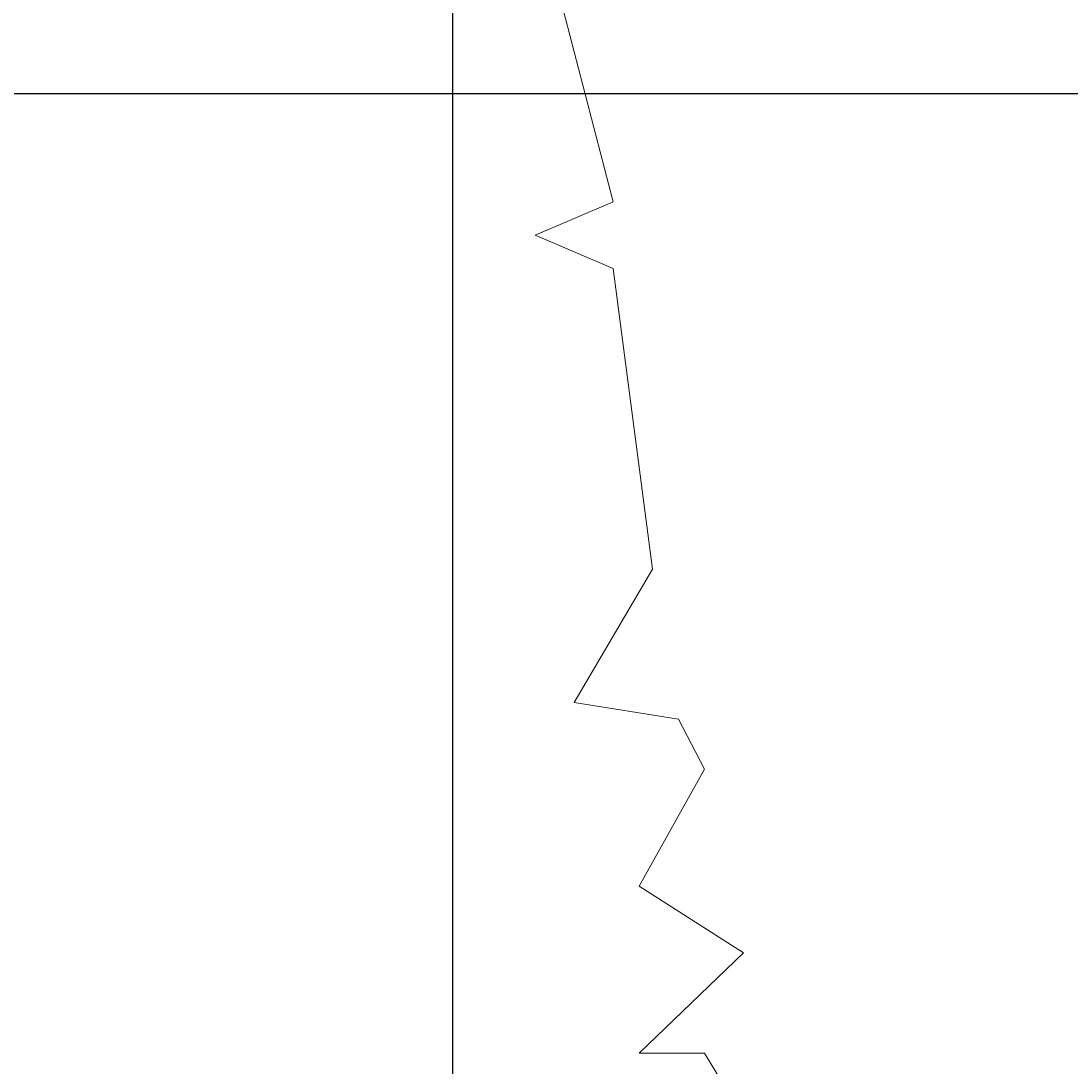
# Model space of a CAD drawing. Units: inches. Extents: x -26 to 776, y -22 to 650.
# Tile 57 of 62: x 506 to 601, y 226 to 321. Entities that reach past the tile are written whole.
import ezdxf

# ---------------------------------------------------------------- set-up
doc = ezdxf.new("R2010")
doc.units = ezdxf.units.IN
doc.header["$MEASUREMENT"] = 0
doc.layers.add('A-ANNO-DIMS', color=2, linetype='Continuous', lineweight=18)
doc.layers.add('L-PLNT-TREE', color=94, linetype='Continuous', lineweight=18)
doc.styles.get("Standard").update_dxf_attribs({"font": 'arial.ttf'})
doc.dimstyles.get("Standard").update_dxf_attribs({"dimtxt": 0.5625, "dimasz": 0.18, "dimexe": 0.18, "dimexo": 0.0625, "dimgap": 0.09, "dimtad": 0, "dimtih": 1, "dimtoh": 1, "dimdec": 4, "dimzin": 0, "dimdsep": 46, "dimlunit": 4, "dimtxsty": 'Standard', "dimcen": 0.09, "dimadec": 0, "dimazin": 0, "dimtfac": 1, "dimtdec": 4, "dimtofl": 0, "dimtmove": 0, "dimatfit": 3, "dimfxl": 1, "dimtolj": 1, "dimtzin": 0, "dimarcsym": 0})

# ---------------------------------------------------------------- blocks, each defined once
blk = doc.blocks.new('Tree - type 2 deciduous elevation')
blk.add_lwpolyline([(34.628, 89.951), (26.576, 103.222), (23.701, 103.222), (28.302, 107.646), (23.701, 110.595), (26.576, 115.756), (25.426, 117.968), (20.825, 118.706), (24.276, 124.604), (22.551, 137.876), (19.1, 139.35), (22.551, 140.825), (19.675, 151.884)])
blk = doc.blocks.new('*D20')
at = {"layer": 'A-ANNO-DIMS', "color": 0, "lineweight": -2, "transparency": 16777216}
for p, q in [((425.806, 455.472), (775.335, 455.472)), ((775.155, 455.292), (775.155, 235.854)), ((775.155, 15.662), (775.155, 235.1)), ((425.806, 15.482), (775.335, 15.482))]:
    blk.add_line(p, q, dxfattribs=at)
at = {"layer": 'A-ANNO-DIMS', "color": 0, "transparency": 16777216}
for points in [[(775.125, 455.292), (775.185, 455.292), (775.155, 455.472)], [(775.125, 15.662), (775.185, 15.662), (775.155, 15.482)]]:
    blk.add_solid(points, dxfattribs=at)
at = {"layer": 'Defpoints', "color": 0, "transparency": 16777216}
for p in [(425.743, 455.472), (775.155, 455.472), (425.743, 15.482)]:
    blk.add_point(p, dxfattribs=at)
at = {"layer": 'A-ANNO-DIMS', "color": 0, "transparency": 16777216, "insert": (775.155, 235.477), "char_height": 0.5625, "attachment_point": 5}
blk.add_mtext('\\A1;440', dxfattribs=at)
blk = doc.blocks.new('*D28')
at = {"layer": 'A-ANNO-DIMS', "color": 0, "lineweight": -2, "transparency": 16777216}
for p, q in [((285.08, 314.119), (775.335, 314.119)), ((775.155, 313.939), (775.155, 243.141)), ((775.155, 171.597), (775.155, 242.396)), ((285.08, 171.417), (775.335, 171.417))]:
    blk.add_line(p, q, dxfattribs=at)
at = {"layer": 'A-ANNO-DIMS', "color": 0, "transparency": 16777216}
for points in [[(775.125, 313.939), (775.185, 313.939), (775.155, 314.119)], [(775.125, 171.597), (775.185, 171.597), (775.155, 171.417)]]:
    blk.add_solid(points, dxfattribs=at)
at = {"layer": 'Defpoints', "color": 0, "transparency": 16777216}
for p in [(285.018, 314.119), (775.155, 314.119), (285.018, 171.417)]:
    blk.add_point(p, dxfattribs=at)
at = {"layer": 'A-ANNO-DIMS', "color": 0, "transparency": 16777216, "insert": (775.155, 242.768), "char_height": 0.5625, "attachment_point": 5}
blk.add_mtext('\\A1;142.7', dxfattribs=at)
blk = doc.blocks.new('*D45')
at = {"layer": 'A-ANNO-DIMS', "color": 0, "lineweight": -2, "transparency": 16777216}
for p, q in [((507.738, 408.639), (775.335, 408.639)), ((775.155, 408.459), (775.155, 212.438)), ((775.155, 15.662), (775.155, 211.683)), ((585.998, 15.482), (775.335, 15.482))]:
    blk.add_line(p, q, dxfattribs=at)
at = {"layer": 'A-ANNO-DIMS', "color": 0, "transparency": 16777216}
for points in [[(775.125, 408.459), (775.185, 408.459), (775.155, 408.639)], [(775.125, 15.662), (775.185, 15.662), (775.155, 15.482)]]:
    blk.add_solid(points, dxfattribs=at)
at = {"layer": 'Defpoints', "color": 0, "transparency": 16777216}
for p in [(507.676, 408.639), (775.155, 408.639), (585.935, 15.482)]:
    blk.add_point(p, dxfattribs=at)
at = {"layer": 'A-ANNO-DIMS', "color": 0, "transparency": 16777216, "insert": (775.155, 212.061), "char_height": 0.5625, "attachment_point": 5}
blk.add_mtext('\\A1;393.16', dxfattribs=at)
blk = doc.blocks.new('*D48')
at = {"layer": 'A-ANNO-DIMS', "color": 0, "lineweight": -2, "transparency": 16777216}
for p, q in [((545.033, 67.415), (545.033, 649.856)), ((545.213, 649.676), (640.879, 649.676)), ((738.57, 649.676), (642.904, 649.676)), ((738.75, 50.911), (738.75, 649.856))]:
    blk.add_line(p, q, dxfattribs=at)
at = {"layer": 'A-ANNO-DIMS', "color": 0, "transparency": 16777216}
for points in [[(545.213, 649.706), (545.213, 649.646), (545.033, 649.676)], [(738.57, 649.706), (738.57, 649.646), (738.75, 649.676)]]:
    blk.add_solid(points, dxfattribs=at)
at = {"layer": 'Defpoints', "color": 0, "transparency": 16777216}
for p in [(738.75, 649.676), (545.033, 67.352), (738.75, 50.848)]:
    blk.add_point(p, dxfattribs=at)
at = {"layer": 'A-ANNO-DIMS', "color": 0, "transparency": 16777216, "insert": (641.892, 649.676), "char_height": 0.5625, "attachment_point": 5}
blk.add_mtext('\\A1;193.7', dxfattribs=at)

msp = doc.modelspace()

# ---------------------------------------------------------------- block references
at = {"layer": 'L-PLNT-TREE', "xscale": 2.050905272406618, "yscale": 2.050905272406618, "zscale": 2.050905272406618}
msp.add_blockref('Tree - type 2 deciduous elevation', (513.3241, 15.4824), dxfattribs=at)

# ---------------------------------------------------------------- dimensions: what is measured, and where the dimension line sits
at = {"layer": 'A-ANNO-DIMS'}
dim = msp.add_linear_dim(base=(738.7503, 649.6763), p1=(545.0331, 67.3523), p2=(738.7503, 50.8482), dimstyle='Standard', override={"dimdec": 1, "dimlfac": 1, "dimrnd": 0, "dimzin": 0, "dimdsep": 46, "dimlunit": 2}, dxfattribs=at)
dim.commit()
dim.dimension.update_dxf_attribs({"geometry": '*D48', "text_midpoint": (641.8917, 649.6763)})
for base, p1, p2, override, picture, middle in [((775.1553, 455.4717), (425.7434, 15.4824), (425.7434, 455.4717), {"dimdec": 0, "dimlfac": 1, "dimrnd": 0, "dimzin": 0, "dimdsep": 46, "dimlunit": 2}, '*D20', (775.1553, 235.477)), ((775.1553, 408.6389), (585.9354, 15.4824), (507.6759, 408.6389), {"dimdec": 2, "dimlfac": 1, "dimrnd": 0, "dimzin": 0, "dimdsep": 46, "dimlunit": 2}, '*D45', (775.1553, 212.0606)), ((775.1553, 314.119), (285.0179, 171.4173), (285.0179, 314.119), {"dimdec": 1, "dimlfac": 1, "dimrnd": 0, "dimzin": 0, "dimdsep": 46, "dimlunit": 2}, '*D28', (775.1553, 242.7682))]:
    dim = msp.add_linear_dim(base=base, p1=p1, p2=p2, angle=90, dimstyle='Standard', override=override, dxfattribs=at)
    dim.commit()
    dim.dimension.update_dxf_attribs({"geometry": picture, "text_midpoint": middle})

doc.saveas('drawing.dxf')
